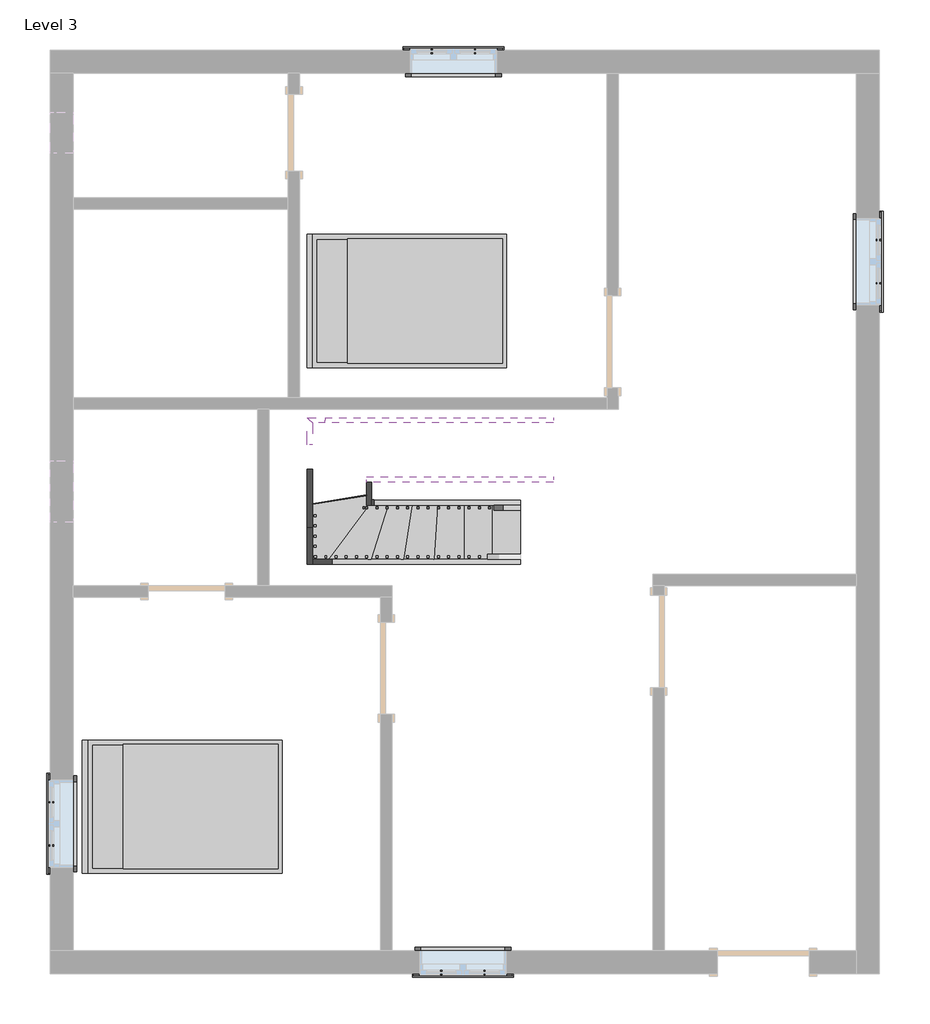
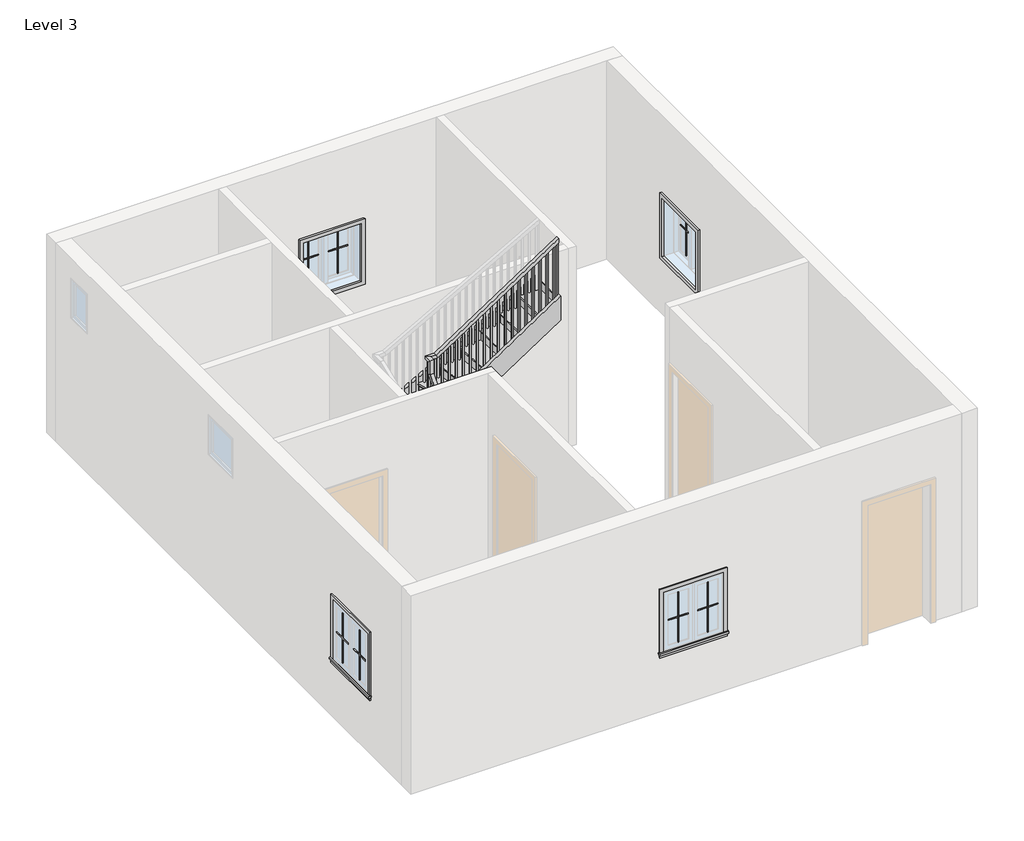
# One storey, part 2 of 2: 16 proxies, 9 members, 2 furniture elements, 1 railing, 1 stair flight.
"""IFC4 building model written with IfcOpenShell, lengths in millimetres."""

from ifc_helpers import new_model, si_unit, frame, origin, place, context, project, spatial, polyline, outline, extrude, faceted_brep, transform, mapped, element, save
from components import muntin_pattern_2x2_muntin_pattern_2x2_b3fe6957, muntin_pattern_2x2_muntin_pattern_2x2_3e0ecaf2, trim_window_exterior_flat_with_sill_41619996, trim_window_interior_flat_picture_frame_51c85655, bed_17739_bed_17739_15c61121, stair_flight_959e1ed9

model = new_model("IFC4")

# Units and contexts
model_context = context("Model", 3, world=origin())
ifc_project = project(units=[si_unit("LENGTHUNIT", "METRE", prefix="MILLI")], contexts=[model_context])

# Site, building, storey
site = spatial("IfcSite", under=ifc_project)
building = spatial("IfcBuilding", under=site)
storey = spatial("IfcBuildingStorey", under=building, Name="Level 3", Elevation=3200.4)

# Proxies
placement = place(None, origin())
muntin_pattern_2x2_muntin_pattern_2x2_shape = muntin_pattern_2x2_muntin_pattern_2x2_b3fe6957(model_context)
element("IfcBuildingElementProxy", 1, Name="Muntin Pattern_2x2 : Muntin Pattern_2x2", ObjectType="Muntin Pattern_2x2 : Muntin Pattern_2x2", at=placement, inside=storey, context=model_context, shape_type="MappedRepresentation", body=[
    mapped(muntin_pattern_2x2_muntin_pattern_2x2_shape, transform((-1143.3273498, 4766.5933073, 4184.65), x_axis=(1.0, 0.0, 0.0), y_axis=(0.0, 1.0, 0.0), z_axis=(0.0, 0.0, 1.0))),
])
element("IfcBuildingElementProxy", 2, Name="Muntin Pattern_2x2 : Muntin Pattern_2x2", ObjectType="Muntin Pattern_2x2 : Muntin Pattern_2x2", at=placement, inside=storey, context=model_context, shape_type="MappedRepresentation", body=[
    mapped(muntin_pattern_2x2_muntin_pattern_2x2_shape, transform((3290.5601502, 2894.9308073, 4184.65), x_axis=(0.0, -1.0, 0.0), y_axis=(1.0, 0.0, 0.0), z_axis=(0.0, 0.0, 1.0))),
])
element("IfcBuildingElementProxy", 3, Name="Muntin Pattern_2x2 : Muntin Pattern_2x2", ObjectType="Muntin Pattern_2x2 : Muntin Pattern_2x2", at=placement, inside=storey, context=model_context, shape_type="MappedRepresentation", body=[
    mapped(muntin_pattern_2x2_muntin_pattern_2x2_shape, transform((-619.4523498, -4374.2316927, 4184.65), x_axis=(-1.0, 0.0, 0.0), y_axis=(0.0, -1.0, 0.0), z_axis=(0.0, 0.0, 1.0))),
])
element("IfcBuildingElementProxy", 4, Name="Muntin Pattern_2x2 : Muntin Pattern_2x2", ObjectType="Muntin Pattern_2x2 : Muntin Pattern_2x2", at=placement, inside=storey, context=model_context, shape_type="MappedRepresentation", body=[
    mapped(muntin_pattern_2x2_muntin_pattern_2x2_shape, transform((-4919.9898498, -3112.1691927, 4184.65), x_axis=(0.0, 1.0, 0.0), y_axis=(-1.0, 0.0, 0.0), z_axis=(0.0, 0.0, 1.0))),
])
muntin_pattern_2x2_muntin_pattern_2x2_2_shape = muntin_pattern_2x2_muntin_pattern_2x2_3e0ecaf2(model_context)
element("IfcBuildingElementProxy", 5, Name="Muntin Pattern_2x2 : Muntin Pattern_2x2", ObjectType="Muntin Pattern_2x2 : Muntin Pattern_2x2", at=placement, inside=storey, context=model_context, shape_type="MappedRepresentation", body=[
    mapped(muntin_pattern_2x2_muntin_pattern_2x2_2_shape, transform((-714.7023498, 4766.5933073, 4184.65), x_axis=(-1.0, 0.0, 0.0), y_axis=(0.0, -1.0, 0.0), z_axis=(0.0, 0.0, 1.0))),
])
element("IfcBuildingElementProxy", 6, Name="Muntin Pattern_2x2 : Muntin Pattern_2x2", ObjectType="Muntin Pattern_2x2 : Muntin Pattern_2x2", at=placement, inside=storey, context=model_context, shape_type="MappedRepresentation", body=[
    mapped(muntin_pattern_2x2_muntin_pattern_2x2_2_shape, transform((3290.5601502, 2466.3058073, 4184.65), x_axis=(0.0, 1.0, 0.0), y_axis=(-1.0, 0.0, 0.0), z_axis=(0.0, 0.0, 1.0))),
])
element("IfcBuildingElementProxy", 7, Name="Muntin Pattern_2x2 : Muntin Pattern_2x2", ObjectType="Muntin Pattern_2x2 : Muntin Pattern_2x2", at=placement, inside=storey, context=model_context, shape_type="MappedRepresentation", body=[
    mapped(muntin_pattern_2x2_muntin_pattern_2x2_2_shape, transform((-1048.0773498, -4374.2316927, 4184.65), x_axis=(1.0, 0.0, 0.0), y_axis=(0.0, 1.0, 0.0), z_axis=(0.0, 0.0, 1.0))),
])
element("IfcBuildingElementProxy", 8, Name="Muntin Pattern_2x2 : Muntin Pattern_2x2", ObjectType="Muntin Pattern_2x2 : Muntin Pattern_2x2", at=placement, inside=storey, context=model_context, shape_type="MappedRepresentation", body=[
    mapped(muntin_pattern_2x2_muntin_pattern_2x2_2_shape, transform((-4919.9898498, -2683.5441927, 4184.65), x_axis=(0.0, -1.0, 0.0), y_axis=(1.0, 0.0, 0.0), z_axis=(0.0, 0.0, 1.0))),
])
trim_window_exterior_flat_with_sill_shape = trim_window_exterior_flat_with_sill_41619996(model_context)
element("IfcBuildingElementProxy", 9, Name="Trim-Window-Exterior-Flat : with Sill", ObjectType="Trim-Window-Exterior-Flat : with Sill", at=placement, inside=storey, context=model_context, shape_type="MappedRepresentation", body=[
    mapped(trim_window_exterior_flat_with_sill_shape, transform((-929.0148498, 4776.1183073, 5029.2), x_axis=(-1.0, 0.0, 0.0), y_axis=(0.0, 0.0, 1.0), z_axis=(0.0, 1.0, 0.0))),
])
element("IfcBuildingElementProxy", 10, Name="Trim-Window-Exterior-Flat : with Sill", ObjectType="Trim-Window-Exterior-Flat : with Sill", at=placement, inside=storey, context=model_context, shape_type="MappedRepresentation", body=[
    mapped(trim_window_exterior_flat_with_sill_shape, transform((3300.0851502, 2680.6183073, 5029.2), x_axis=(0.0, 1.0, 0.0), y_axis=(0.0, 0.0, 1.0), z_axis=(1.0, 0.0, 0.0))),
])
element("IfcBuildingElementProxy", 11, Name="Trim-Window-Exterior-Flat : with Sill", ObjectType="Trim-Window-Exterior-Flat : with Sill", at=placement, inside=storey, context=model_context, shape_type="MappedRepresentation", body=[
    mapped(trim_window_exterior_flat_with_sill_shape, transform((-833.7648498, -4383.7566927, 5029.2), x_axis=(1.0, 0.0, 0.0), y_axis=(0.0, 0.0, 1.0), z_axis=(0.0, -1.0, 0.0))),
])
element("IfcBuildingElementProxy", 12, Name="Trim-Window-Exterior-Flat : with Sill", ObjectType="Trim-Window-Exterior-Flat : with Sill", at=placement, inside=storey, context=model_context, shape_type="MappedRepresentation", body=[
    mapped(trim_window_exterior_flat_with_sill_shape, transform((-4929.5148498, -2897.8566927, 5029.2), x_axis=(0.0, -1.0, 0.0), y_axis=(0.0, 0.0, 1.0), z_axis=(-1.0, 0.0, 0.0))),
])
trim_window_interior_flat_picture_frame_shape = trim_window_interior_flat_picture_frame_51c85655(model_context)
element("IfcBuildingElementProxy", 13, Name="Trim-Window-Interior-Flat : Picture Frame", ObjectType="Trim-Window-Interior-Flat : Picture Frame", at=placement, inside=storey, context=model_context, shape_type="MappedRepresentation", body=[
    mapped(trim_window_interior_flat_picture_frame_shape, transform((-929.0148498, 4547.5183073, 5029.2), x_axis=(1.0, 0.0, 0.0), y_axis=(0.0, 0.0, 1.0), z_axis=(0.0, -1.0, 0.0))),
])
element("IfcBuildingElementProxy", 14, Name="Trim-Window-Interior-Flat : Picture Frame", ObjectType="Trim-Window-Interior-Flat : Picture Frame", at=placement, inside=storey, context=model_context, shape_type="MappedRepresentation", body=[
    mapped(trim_window_interior_flat_picture_frame_shape, transform((3071.4851502, 2680.6183073, 5029.2), x_axis=(0.0, -1.0, 0.0), y_axis=(0.0, 0.0, 1.0), z_axis=(-1.0, 0.0, 0.0))),
])
element("IfcBuildingElementProxy", 15, Name="Trim-Window-Interior-Flat : Picture Frame", ObjectType="Trim-Window-Interior-Flat : Picture Frame", at=placement, inside=storey, context=model_context, shape_type="MappedRepresentation", body=[
    mapped(trim_window_interior_flat_picture_frame_shape, transform((-833.7648498, -4155.1566927, 5029.2), x_axis=(-1.0, 0.0, 0.0), y_axis=(0.0, 0.0, 1.0), z_axis=(0.0, 1.0, 0.0))),
])
element("IfcBuildingElementProxy", 16, Name="Trim-Window-Interior-Flat : Picture Frame", ObjectType="Trim-Window-Interior-Flat : Picture Frame", at=placement, inside=storey, context=model_context, shape_type="MappedRepresentation", body=[
    mapped(trim_window_interior_flat_picture_frame_shape, transform((-4700.9148498, -2897.8566927, 5029.2), x_axis=(0.0, 1.0, 0.0), y_axis=(0.0, 0.0, 1.0), z_axis=(1.0, 0.0, 0.0))),
])

# Furniture
bed_17739_bed_17739_shape = bed_17739_bed_17739_15c61121(model_context)
element("IfcFurniture", 17, ObjectType="Bed_17739 : Bed_17739", at=placement, inside=storey, context=model_context, shape_type="MappedRepresentation", body=[
    mapped(bed_17739_bed_17739_shape, transform((-3596.0148498, -2726.4066927, 3200.4), x_axis=(0.0, 1.0, 0.0), y_axis=(-1.0, 0.0, 0.0), z_axis=(0.0, 0.0, 1.0))),
])
element("IfcFurniture", 18, ObjectType="Bed_17739 : Bed_17739", at=placement, inside=storey, context=model_context, shape_type="MappedRepresentation", body=[
    mapped(bed_17739_bed_17739_shape, transform((-1367.1648498, 2290.0933073, 3200.4), x_axis=(0.0, 1.0, 0.0), y_axis=(-1.0, 0.0, 0.0), z_axis=(0.0, 0.0, 1.0))),
])

# Members
element("IfcMember", 19, ObjectType="Stringer - 2\" Width", at=placement, inside=storey, context=model_context, shape_type="SweptSolid", body=[
    extrude(outline(polyline([(3200.4, -264.8831579), (3428.8652135, -264.8831579), (4504.6576628, -2328.8610857), (4160.9393024, -2328.8610857), (3200.4, -486.0038318), (3200.4, -264.8831579)])), frame((0.0, -322.6029286, 0.0), z_axis=(0.0, 1.0, 0.0), x_axis=(0.0, 0.0, 1.0)), (0.0, 0.0, 1.0), 50.8),
])
element("IfcMember", 20, ObjectType="Stringer - 2\" Width", at=placement, inside=storey, context=model_context, shape_type="SweptSolid", body=[
    extrude(outline(polyline([(-2328.8610857, -322.6029286), (-2379.6610857, -322.6029286), (-2379.6610857, 39.7116887), (-2328.8610857, 39.7116887), (-2328.8610857, -322.6029286)])), frame((0.0, 0.0, 4160.9393024), z_axis=(0.0, 0.0, 1.0), x_axis=(1.0, 0.0, 0.0)), (0.0, 0.0, 1.0), 343.7183604),
])
element("IfcMember", 21, ObjectType="Stringer - 2\" Width", at=placement, inside=storey, context=model_context, shape_type="SweptSolid", body=[
    extrude(outline(polyline([(39.7116887, 4160.9393024), (39.7116887, 4504.6576628), (861.172384, 4844.4948766), (861.172384, 4500.7765162), (39.7116887, 4160.9393024)])), frame((-2379.6610857, 0.0, 0.0), z_axis=(1.0, 0.0, 0.0), x_axis=(0.0, 1.0, 0.0)), (0.0, 0.0, 1.0), 50.8),
])
element("IfcMember", 22, ObjectType="Stringer - 2\" Width", at=placement, inside=storey, context=model_context, shape_type="SweptSolid", body=[
    extrude(outline(polyline([(-2328.8610857, 861.172384), (-2379.6610857, 861.172384), (-2379.6610857, 1130.8895433), (-2328.8610857, 1080.0895433), (-2328.8610857, 861.172384)])), frame((0.0, 0.0, 4507.0790002), z_axis=(0.0, 0.0, 1.0), x_axis=(1.0, 0.0, 0.0)), (0.0, 0.0, 1.0), 329.8531189),
])
element("IfcMember", 23, ObjectType="Stringer - 2\" Width", at=placement, inside=storey, context=model_context, shape_type="SweptSolid", body=[
    extrude(outline(polyline([(-2328.8610857, 1080.0895433), (-2379.6610857, 1130.8895433), (-2203.9193363, 1130.8895433), (-2203.9193363, 1080.0895433), (-2328.8610857, 1080.0895433)])), frame((0.0, 0.0, 4507.0790002), z_axis=(0.0, 0.0, 1.0), x_axis=(1.0, 0.0, 0.0)), (0.0, 0.0, 1.0), 329.8531189),
])
element("IfcMember", 24, ObjectType="Stringer - 2\" Width", at=placement, inside=storey, context=model_context, shape_type="SweptSolid", body=[
    extrude(outline(polyline([(3200.4, -264.8831579), (3397.3581828, -264.8831579), (4416.8545254, -1741.8148498), (4046.4897368, -1741.8148498), (3200.4, -516.0951544), (3200.4, -264.8831579)])), frame((0.0, 264.4433073, 0.0), z_axis=(0.0, 1.0, 0.0), x_axis=(0.0, 0.0, 1.0)), (0.0, 0.0, 1.0), 50.8),
])
element("IfcMember", 25, ObjectType="Stringer - 2\" Width", at=placement, inside=storey, context=model_context, shape_type="SweptSolid", body=[
    extrude(outline(polyline([(264.4433073, 4126.1590756), (264.4433073, 4585.358282), (493.0433073, 4842.9490234), (493.0433073, 4383.749817), (264.4433073, 4126.1590756)])), frame((-1792.6148498, 0.0, 0.0), z_axis=(1.0, 0.0, 0.0), x_axis=(0.0, 1.0, 0.0)), (0.0, 0.0, 1.0), 50.8),
])
element("IfcMember", 26, ObjectType="Stringer - 2\" Width", at=placement, inside=storey, context=model_context, shape_type="SweptSolid", body=[
    extrude(outline(polyline([(4916.0438732, -1792.6148498), (4550.7121415, -1792.6148498), (5777.1313098, 63.4034409), (6142.4630415, 63.4034409), (4916.0438732, -1792.6148498)])), frame((0.0, 493.0433073, 0.0), z_axis=(0.0, 1.0, 0.0), x_axis=(0.0, 0.0, 1.0)), (0.0, 0.0, 1.0), 50.8),
])
element("IfcMember", 27, ObjectType="Stringer - 2\" Width", at=placement, inside=storey, context=model_context, shape_type="SweptSolid", body=[
    extrude(outline(polyline([(4836.932119, -2203.9193363), (4507.0790002, -2203.9193363), (5762.442957, 63.4034409), (6092.2960758, 63.4034409), (4836.932119, -2203.9193363)])), frame((0.0, 1080.0895433, 0.0), z_axis=(0.0, 1.0, 0.0), x_axis=(0.0, 0.0, 1.0)), (0.0, 0.0, 1.0), 50.8),
])

# Railing
element("IfcRailing", 28, ObjectType="Handrail - Rectangular", at=placement, inside=storey, context=model_context, shape_type="SolidModel", body=[
    faceted_brep([(-264.8831579, 213.6433073, 4284.1333333), (-264.8831579, 213.6433073, 4222.8533076), (-264.8831579, 264.4433073, 4222.8533076), (-264.8831579, 264.4433073, 4284.1333333), (-1716.4148498, 213.6433073, 5263.4160626), (-1767.2148498, 213.6433073, 5236.4084974), (-1767.2148498, 264.4433073, 5236.4084974), (-1716.4148498, 264.4433073, 5263.4160626), (-1716.4148498, 213.6433073, 5477.9989826), (-1767.2148498, 213.6433073, 5427.1989826), (-1767.2148498, 264.4433073, 5427.1989826), (-1716.4148498, 264.4433073, 5477.9989826), (-1843.4148498, 213.6433073, 5477.9989826), (-1843.4148498, 213.6433073, 5427.1989826), (-1792.6148498, 264.4433073, 5427.1989826), (-1792.6148498, 264.4433073, 5477.9989826), (-1843.4148498, 340.6433073, 5477.9989826), (-1843.4148498, 363.4803462, 5427.1989826), (-1792.6148498, 363.4803462, 5427.1989826), (-1792.6148498, 340.6433073, 5477.9989826), (-1843.4148498, 467.6433073, 5621.10495), (-1843.4148498, 518.4433073, 5601.8141359), (-1792.6148498, 518.4433073, 5601.8141359), (-1792.6148498, 467.6433073, 5621.10495), (-1843.4148498, 467.6433073, 5832.374751), (-1843.4148498, 518.4433073, 5781.574751), (-1792.6148498, 518.4433073, 5781.574751), (-1792.6148498, 467.6433073, 5832.374751), (-1843.4148498, 594.6433073, 5832.374751), (-1843.4148498, 594.6433073, 5781.574751), (-1792.6148498, 543.8433073, 5781.574751), (-1792.6148498, 543.8433073, 5832.374751), (-1716.4148498, 594.6433073, 5832.374751), (-1701.3097842, 594.6433073, 5781.574751), (-1701.3097842, 543.8433073, 5781.574751), (-1716.4148498, 543.8433073, 5832.374751), (63.4034409, 594.6433073, 6993.4666667), (63.4034409, 543.8433073, 6993.4666667), (63.4034409, 543.8433073, 6932.8126442), (63.4034409, 594.6433073, 6932.8126442)], [[[0, 1, 2, 3]], [[1, 0, 4, 5]], [[2, 1, 5, 6]], [[3, 2, 6, 7]], [[0, 3, 7, 4]], [[5, 4, 8, 9]], [[6, 5, 9, 10]], [[7, 6, 10, 11]], [[4, 7, 11, 8]], [[9, 8, 12, 13]], [[10, 9, 13, 14]], [[11, 10, 14, 15]], [[8, 11, 15, 12]], [[13, 12, 16, 17]], [[14, 13, 17, 18]], [[15, 14, 18, 19]], [[12, 15, 19, 16]], [[17, 16, 20, 21]], [[18, 17, 21, 22]], [[19, 18, 22, 23]], [[16, 19, 23, 20]], [[21, 20, 24, 25]], [[22, 21, 25, 26]], [[23, 22, 26, 27]], [[20, 23, 27, 24]], [[25, 24, 28, 29]], [[26, 25, 29, 30]], [[27, 26, 30, 31]], [[24, 27, 31, 28]], [[29, 28, 32, 33]], [[30, 29, 33, 34]], [[31, 30, 34, 35]], [[28, 31, 35, 32]], [[36, 37, 38, 39]], [[33, 32, 36, 39]], [[34, 33, 39, 38]], [[35, 34, 38, 37]], [[32, 35, 37, 36]]]),
    extrude(outline(polyline([(6904.7000713, 20.3101502), (6892.27251, 1.2601502), (5909.7333333, 1.2601502), (5909.7333333, 20.3101502), (6904.7000713, 20.3101502)])), frame((0.0, 559.7183073, 0.0), z_axis=(0.0, 1.0, 0.0), x_axis=(0.0, 0.0, 1.0)), (0.0, 0.0, 1.0), 19.05),
    extrude(outline(polyline([(6838.4197441, -81.2898498), (6825.9921828, -100.3398498), (5909.7333333, -100.3398498), (5909.7333333, -81.2898498), (6838.4197441, -81.2898498)])), frame((0.0, 559.7183073, 0.0), z_axis=(0.0, 1.0, 0.0), x_axis=(0.0, 0.0, 1.0)), (0.0, 0.0, 1.0), 19.05),
    extrude(outline(polyline([(6772.139417, -182.8898498), (6759.7118556, -201.9398498), (5909.7333333, -201.9398498), (5909.7333333, -182.8898498), (6772.139417, -182.8898498)])), frame((0.0, 559.7183073, 0.0), z_axis=(0.0, 1.0, 0.0), x_axis=(0.0, 0.0, 1.0)), (0.0, 0.0, 1.0), 19.05),
    extrude(outline(polyline([(6705.8590898, -284.4898498), (6693.4315284, -303.5398498), (5740.4, -303.5398498), (5740.4, -284.4898498), (6705.8590898, -284.4898498)])), frame((0.0, 559.7183073, 0.0), z_axis=(0.0, 1.0, 0.0), x_axis=(0.0, 0.0, 1.0)), (0.0, 0.0, 1.0), 19.05),
    extrude(outline(polyline([(6639.5787626, -386.0898498), (6627.1512012, -405.1398498), (5740.4, -405.1398498), (5740.4, -386.0898498), (6639.5787626, -386.0898498)])), frame((0.0, 559.7183073, 0.0), z_axis=(0.0, 1.0, 0.0), x_axis=(0.0, 0.0, 1.0)), (0.0, 0.0, 1.0), 19.05),
    extrude(outline(polyline([(6573.2984354, -487.6898498), (6560.8708741, -506.7398498), (5571.0666667, -506.7398498), (5571.0666667, -487.6898498), (6573.2984354, -487.6898498)])), frame((0.0, 559.7183073, 0.0), z_axis=(0.0, 1.0, 0.0), x_axis=(0.0, 0.0, 1.0)), (0.0, 0.0, 1.0), 19.05),
    extrude(outline(polyline([(6507.0181082, -589.2898498), (6494.5905469, -608.3398498), (5571.0666667, -608.3398498), (5571.0666667, -589.2898498), (6507.0181082, -589.2898498)])), frame((0.0, 559.7183073, 0.0), z_axis=(0.0, 1.0, 0.0), x_axis=(0.0, 0.0, 1.0)), (0.0, 0.0, 1.0), 19.05),
    extrude(outline(polyline([(6440.7377811, -690.8898498), (6428.3102197, -709.9398498), (5571.0666667, -709.9398498), (5571.0666667, -690.8898498), (6440.7377811, -690.8898498)])), frame((0.0, 559.7183073, 0.0), z_axis=(0.0, 1.0, 0.0), x_axis=(0.0, 0.0, 1.0)), (0.0, 0.0, 1.0), 19.05),
    extrude(outline(polyline([(6374.4574539, -792.4898498), (6362.0298925, -811.5398498), (5401.7333333, -811.5398498), (5401.7333333, -792.4898498), (6374.4574539, -792.4898498)])), frame((0.0, 559.7183073, 0.0), z_axis=(0.0, 1.0, 0.0), x_axis=(0.0, 0.0, 1.0)), (0.0, 0.0, 1.0), 19.05),
    extrude(outline(polyline([(6308.1771267, -894.0898498), (6295.7495653, -913.1398498), (5401.7333333, -913.1398498), (5401.7333333, -894.0898498), (6308.1771267, -894.0898498)])), frame((0.0, 559.7183073, 0.0), z_axis=(0.0, 1.0, 0.0), x_axis=(0.0, 0.0, 1.0)), (0.0, 0.0, 1.0), 19.05),
    extrude(outline(polyline([(6241.8967995, -995.6898498), (6229.4692382, -1014.7398498), (5401.7333333, -1014.7398498), (5401.7333333, -995.6898498), (6241.8967995, -995.6898498)])), frame((0.0, 559.7183073, 0.0), z_axis=(0.0, 1.0, 0.0), x_axis=(0.0, 0.0, 1.0)), (0.0, 0.0, 1.0), 19.05),
    extrude(outline(polyline([(6175.6164723, -1097.2898498), (6163.188911, -1116.3398498), (5232.4, -1116.3398498), (5232.4, -1097.2898498), (6175.6164723, -1097.2898498)])), frame((0.0, 559.7183073, 0.0), z_axis=(0.0, 1.0, 0.0), x_axis=(0.0, 0.0, 1.0)), (0.0, 0.0, 1.0), 19.05),
    extrude(outline(polyline([(6109.3361451, -1198.8898498), (6096.9085838, -1217.9398498), (5232.4, -1217.9398498), (5232.4, -1198.8898498), (6109.3361451, -1198.8898498)])), frame((0.0, 559.7183073, 0.0), z_axis=(0.0, 1.0, 0.0), x_axis=(0.0, 0.0, 1.0)), (0.0, 0.0, 1.0), 19.05),
    extrude(outline(polyline([(6043.055818, -1300.4898498), (6030.6282566, -1319.5398498), (5063.0666667, -1319.5398498), (5063.0666667, -1300.4898498), (6043.055818, -1300.4898498)])), frame((0.0, 559.7183073, 0.0), z_axis=(0.0, 1.0, 0.0), x_axis=(0.0, 0.0, 1.0)), (0.0, 0.0, 1.0), 19.05),
    extrude(outline(polyline([(5976.7754908, -1402.0898498), (5964.3479294, -1421.1398498), (5063.0666667, -1421.1398498), (5063.0666667, -1402.0898498), (5976.7754908, -1402.0898498)])), frame((0.0, 559.7183073, 0.0), z_axis=(0.0, 1.0, 0.0), x_axis=(0.0, 0.0, 1.0)), (0.0, 0.0, 1.0), 19.05),
    extrude(outline(polyline([(5910.4951636, -1503.6898498), (5898.0676023, -1522.7398498), (5063.0666667, -1522.7398498), (5063.0666667, -1503.6898498), (5910.4951636, -1503.6898498)])), frame((0.0, 559.7183073, 0.0), z_axis=(0.0, 1.0, 0.0), x_axis=(0.0, 0.0, 1.0)), (0.0, 0.0, 1.0), 19.05),
    extrude(outline(polyline([(5844.2148364, -1605.2898498), (5831.7872751, -1624.3398498), (4893.7333333, -1624.3398498), (4893.7333333, -1605.2898498), (5844.2148364, -1605.2898498)])), frame((0.0, 559.7183073, 0.0), z_axis=(0.0, 1.0, 0.0), x_axis=(0.0, 0.0, 1.0)), (0.0, 0.0, 1.0), 19.05),
    extrude(outline(polyline([(5777.9345092, -1706.8898498), (5765.5069479, -1725.9398498), (4893.7333333, -1725.9398498), (4893.7333333, -1706.8898498), (5777.9345092, -1706.8898498)])), frame((0.0, 559.7183073, 0.0), z_axis=(0.0, 1.0, 0.0), x_axis=(0.0, 0.0, 1.0)), (0.0, 0.0, 1.0), 19.05),
    extrude(outline(polyline([(-1808.4898498, 534.3183073), (-1827.5398498, 534.3183073), (-1827.5398498, 553.3683073), (-1808.4898498, 553.3683073), (-1808.4898498, 534.3183073)])), frame((0.0, 0.0, 4724.4), z_axis=(0.0, 0.0, 1.0), x_axis=(1.0, 0.0, 0.0)), (0.0, 0.0, 1.0), 1057.174751),
    extrude(outline(polyline([(432.7183073, 5505.2176079), (451.7683073, 5526.683503), (451.7683073, 4555.0666667), (432.7183073, 4555.0666667), (432.7183073, 5505.2176079)])), frame((-1827.5398498, 0.0, 0.0), z_axis=(1.0, 0.0, 0.0), x_axis=(0.0, 1.0, 0.0)), (0.0, 0.0, 1.0), 19.05),
    extrude(outline(polyline([(331.1183073, 5390.732834), (350.1683073, 5412.1987291), (350.1683073, 4555.0666667), (331.1183073, 4555.0666667), (331.1183073, 5390.732834)])), frame((-1827.5398498, 0.0, 0.0), z_axis=(1.0, 0.0, 0.0), x_axis=(0.0, 1.0, 0.0)), (0.0, 0.0, 1.0), 19.05),
    extrude(outline(polyline([(-1779.3581579, 248.5683073), (-1779.3581579, 229.5183073), (-1798.4081579, 229.5183073), (-1798.4081579, 248.5683073), (-1779.3581579, 248.5683073)])), frame((0.0, 0.0, 4216.4), z_axis=(0.0, 0.0, 1.0), x_axis=(1.0, 0.0, 0.0)), (0.0, 0.0, 1.0), 1210.7989826),
    extrude(outline(polyline([(5176.0561166, -1677.7581579), (5188.9082893, -1696.8081579), (4216.4, -1696.8081579), (4216.4, -1677.7581579), (5176.0561166, -1677.7581579)])), frame((0.0, 229.5183073, 0.0), z_axis=(0.0, 1.0, 0.0), x_axis=(0.0, 0.0, 1.0)), (0.0, 0.0, 1.0), 19.05),
    extrude(outline(polyline([(5107.5111955, -1576.1581579), (5120.3633682, -1595.2081579), (4216.4, -1595.2081579), (4216.4, -1576.1581579), (5107.5111955, -1576.1581579)])), frame((0.0, 229.5183073, 0.0), z_axis=(0.0, 1.0, 0.0), x_axis=(0.0, 0.0, 1.0)), (0.0, 0.0, 1.0), 19.05),
    extrude(outline(polyline([(5038.9662744, -1474.5581579), (5051.8184472, -1493.6081579), (4047.0666667, -1493.6081579), (4047.0666667, -1474.5581579), (5038.9662744, -1474.5581579)])), frame((0.0, 229.5183073, 0.0), z_axis=(0.0, 1.0, 0.0), x_axis=(0.0, 0.0, 1.0)), (0.0, 0.0, 1.0), 19.05),
    extrude(outline(polyline([(4970.4213533, -1372.9581579), (4983.2735261, -1392.0081579), (4047.0666667, -1392.0081579), (4047.0666667, -1372.9581579), (4970.4213533, -1372.9581579)])), frame((0.0, 229.5183073, 0.0), z_axis=(0.0, 1.0, 0.0), x_axis=(0.0, 0.0, 1.0)), (0.0, 0.0, 1.0), 19.05),
    extrude(outline(polyline([(4901.8764322, -1271.3581579), (4914.728605, -1290.4081579), (3877.7333333, -1290.4081579), (3877.7333333, -1271.3581579), (4901.8764322, -1271.3581579)])), frame((0.0, 229.5183073, 0.0), z_axis=(0.0, 1.0, 0.0), x_axis=(0.0, 0.0, 1.0)), (0.0, 0.0, 1.0), 19.05),
    extrude(outline(polyline([(4833.3315111, -1169.7581579), (4846.1836839, -1188.8081579), (3877.7333333, -1188.8081579), (3877.7333333, -1169.7581579), (4833.3315111, -1169.7581579)])), frame((0.0, 229.5183073, 0.0), z_axis=(0.0, 1.0, 0.0), x_axis=(0.0, 0.0, 1.0)), (0.0, 0.0, 1.0), 19.05),
    extrude(outline(polyline([(4764.78659, -1068.1581579), (4777.6387628, -1087.2081579), (3708.4, -1087.2081579), (3708.4, -1068.1581579), (4764.78659, -1068.1581579)])), frame((0.0, 229.5183073, 0.0), z_axis=(0.0, 1.0, 0.0), x_axis=(0.0, 0.0, 1.0)), (0.0, 0.0, 1.0), 19.05),
    extrude(outline(polyline([(4696.241669, -966.5581579), (4709.0938417, -985.6081579), (3708.4, -985.6081579), (3708.4, -966.5581579), (4696.241669, -966.5581579)])), frame((0.0, 229.5183073, 0.0), z_axis=(0.0, 1.0, 0.0), x_axis=(0.0, 0.0, 1.0)), (0.0, 0.0, 1.0), 19.05),
    extrude(outline(polyline([(4627.6967479, -864.9581579), (4640.5489206, -884.0081579), (3708.4, -884.0081579), (3708.4, -864.9581579), (4627.6967479, -864.9581579)])), frame((0.0, 229.5183073, 0.0), z_axis=(0.0, 1.0, 0.0), x_axis=(0.0, 0.0, 1.0)), (0.0, 0.0, 1.0), 19.05),
    extrude(outline(polyline([(4559.1518268, -763.3581579), (4572.0039995, -782.4081579), (3539.0666667, -782.4081579), (3539.0666667, -763.3581579), (4559.1518268, -763.3581579)])), frame((0.0, 229.5183073, 0.0), z_axis=(0.0, 1.0, 0.0), x_axis=(0.0, 0.0, 1.0)), (0.0, 0.0, 1.0), 19.05),
    extrude(outline(polyline([(4490.6069057, -661.7581579), (4503.4590784, -680.8081579), (3539.0666667, -680.8081579), (3539.0666667, -661.7581579), (4490.6069057, -661.7581579)])), frame((0.0, 229.5183073, 0.0), z_axis=(0.0, 1.0, 0.0), x_axis=(0.0, 0.0, 1.0)), (0.0, 0.0, 1.0), 19.05),
    extrude(outline(polyline([(4422.0619846, -560.1581579), (4434.9141573, -579.2081579), (3539.0666667, -579.2081579), (3539.0666667, -560.1581579), (4422.0619846, -560.1581579)])), frame((0.0, 229.5183073, 0.0), z_axis=(0.0, 1.0, 0.0), x_axis=(0.0, 0.0, 1.0)), (0.0, 0.0, 1.0), 19.05),
    extrude(outline(polyline([(4353.5170635, -458.5581579), (4366.3692362, -477.6081579), (3369.7333333, -477.6081579), (3369.7333333, -458.5581579), (4353.5170635, -458.5581579)])), frame((0.0, 229.5183073, 0.0), z_axis=(0.0, 1.0, 0.0), x_axis=(0.0, 0.0, 1.0)), (0.0, 0.0, 1.0), 19.05),
    extrude(outline(polyline([(4284.9721424, -356.9581579), (4297.8243151, -376.0081579), (3369.7333333, -376.0081579), (3369.7333333, -356.9581579), (4284.9721424, -356.9581579)])), frame((0.0, 229.5183073, 0.0), z_axis=(0.0, 1.0, 0.0), x_axis=(0.0, 0.0, 1.0)), (0.0, 0.0, 1.0), 19.05),
    extrude(outline(polyline([(-1808.4898498, 559.7183073), (-1827.5398498, 559.7183073), (-1827.5398498, 578.7683073), (-1808.4898498, 578.7683073), (-1808.4898498, 559.7183073)])), frame((0.0, 0.0, 4724.4), z_axis=(0.0, 0.0, 1.0), x_axis=(1.0, 0.0, 0.0)), (0.0, 0.0, 1.0), 1057.174751),
    extrude(outline(polyline([(-1808.4898498, 248.5683073), (-1808.4898498, 229.5183073), (-1827.5398498, 229.5183073), (-1827.5398498, 248.5683073), (-1808.4898498, 248.5683073)])), frame((0.0, 0.0, 4385.7333333), z_axis=(0.0, 0.0, 1.0), x_axis=(1.0, 0.0, 0.0)), (0.0, 0.0, 1.0), 1041.4656493),
    extrude(outline(polyline([(6932.8126442, 63.4034409), (6920.3850828, 44.3534409), (5909.7333333, 44.3534409), (5909.7333333, 63.4034409), (6932.8126442, 63.4034409)])), frame((0.0, 559.7183073, 0.0), z_axis=(0.0, 1.0, 0.0), x_axis=(0.0, 0.0, 1.0)), (0.0, 0.0, 1.0), 19.05),
    extrude(outline(polyline([(4222.8533076, -264.8831579), (4235.7054803, -283.9331579), (3369.7333333, -283.9331579), (3369.7333333, -264.8831579), (4222.8533076, -264.8831579)])), frame((0.0, 229.5183073, 0.0), z_axis=(0.0, 1.0, 0.0), x_axis=(0.0, 0.0, 1.0)), (0.0, 0.0, 1.0), 19.05),
])

# Stair flight
stair_flight_shape = stair_flight_959e1ed9(model_context)
element("IfcStairFlight", 29, ObjectType="2\" Tread 1\" Nosing 1/4\" Riser", at=placement, inside=storey, context=model_context, shape_type="MappedRepresentation", body=[
    mapped(stair_flight_shape, transform((0.0, 0.0, 0.0), x_axis=(1.0, 0.0, 0.0), y_axis=(0.0, 1.0, 0.0), z_axis=(0.0, 0.0, 1.0))),
])

save(model, "model.ifc")

# Revit data of these elements
# Type "Muntin Pattern_2x2 : Muntin Pattern_2x2"
#   Width [instance default] = 4' - 0"
#   Thickness = 0' - 0 1/2"
#   Height [instance default] = 4' - 0"
#   Distance = 0' - 0 3/4"
#   Interior Material [instance default] = none
#   Exterior Material [instance default] = none
#   Default Elevation = 0
# Type "Trim-Window-Exterior-Flat : with Sill"
#   Trim Width = 0' - 2 1/4"
#   Trim Thickness_Picture Frame = 0' - 1 1/4"
#   Trim Thickness_with Sill = 0' - 0 3/4"
#   Sill Thickness = 0' - 1 1/4"
#   Opening Width [instance default] = 2' - 0"
#   Opening Height [instance default] = 3' - 0"
#   Default Elevation = 4' - 0"
#   Sill = yes
#   Picture Frame = no
#   Trim Material [instance default] = none
# Type "Trim-Window-Interior-Flat : Picture Frame"
#   Trim Thickness_Picture Frame = 0' - 1 1/4"
#   Trim Width = 0' - 2 1/4"
#   Trim Thickness_with Sill = 0' - 0 3/4"
#   Sill Thickness = 0' - 1 1/4"
#   Opening Width [instance default] = 2' - 0"
#   Opening Height [instance default] = 3' - 0"
#   Default Elevation = 4' - 0"
#   Sill = no
#   Picture Frame = yes
#   Trim Material [instance default] = none
# Type "Bed_17739 : Bed_17739"
#   Default Elevation = 0
# Type "Handrail - Rectangular"
#   Assembly Code = "C2010400"
#   built-in parameter 1008612 = 0.0416667 (stored number, unit not read)
#   built-in parameter 1008611 = 0.0416667 (stored number, unit not read)
#   built-in parameter 1008609 = 0.333333 (stored number, unit not read)
#   built-in parameter 1008604 = 0.166667 (stored number, unit not read)
#   built-in parameter 1008603 = 0.166667 (stored number, unit not read)
#   Railing Height = 3' - 0"
#   built-in parameter 1008630 = 2
#   built-in parameter 1008610 = 2
#   built-in parameter 1008618 = Baluster - Square : 3/4"
# Elements 1, 2, 3, 4, 5, 6, 7, 8 (IfcBuildingElementProxy, "Muntin Pattern_2x2 : Muntin Pattern_2x2")
#   Width = 0' - 11 5/8"
#   Height = 2' - 6 1/2"
#   Interior Material = Wood - Stained
#   Exterior Material = Clad - White
#   Phase Created = New Construction
#   Materials on its faces: "Clad - White", "Wood - Stained"
# Elements 9, 10, 11, 12 (IfcBuildingElementProxy, "Trim-Window-Exterior-Flat : with Sill")
#   Opening Width = 2' - 10"
#   Opening Height = 3' - 0"
#   Trim Material = Clad - White
#   Phase Created = New Construction
#   Materials on its faces: "Clad - White"
# Elements 13, 14, 15, 16 (IfcBuildingElementProxy, "Trim-Window-Interior-Flat : Picture Frame")
#   Opening Width = 2' - 10"
#   Opening Height = 3' - 0"
#   Trim Material = Wood - Stained
#   Phase Created = New Construction
#   Materials on its faces: "Wood - Stained"
# Elements 17, 18 (IfcFurniture, "Bed_17739 : Bed_17739")
#   Phase Created = New Construction
#   Materials on its faces: "legs", "sheets", "bed frame", "Blanket"
# Elements 19, 20, 21, 22, 23, 24, 25, 26, 27 (IfcMember, "Stringer - 2\" Width")
#   Phase Created = New Construction
# Element 28 (IfcRailing, "Handrail - Rectangular")
#   Phase Created = New Construction
# Element 29 (IfcStairFlight, "2\" Tread 1\" Nosing 1/4\" Riser")
#   Phase Created = New Construction
# Materials
#   "Clad - White": class "Wood", colour RGB 242 242 238, transparency 0, Cost = 0
#   "Wood - Stained": class "Wood", colour RGB 224 178 126, transparency 0, Cost = 0
#   "legs": colour RGB 90 73 37, transparency 0, Cost = 0
#   "sheets": colour RGB 200 195 176, transparency 0, Cost = 0
#   "bed frame": colour RGB 90 73 37, transparency 0, Cost = 0
#   "Blanket": class "System", colour RGB 59 0 1, transparency 0, Cost = 0
